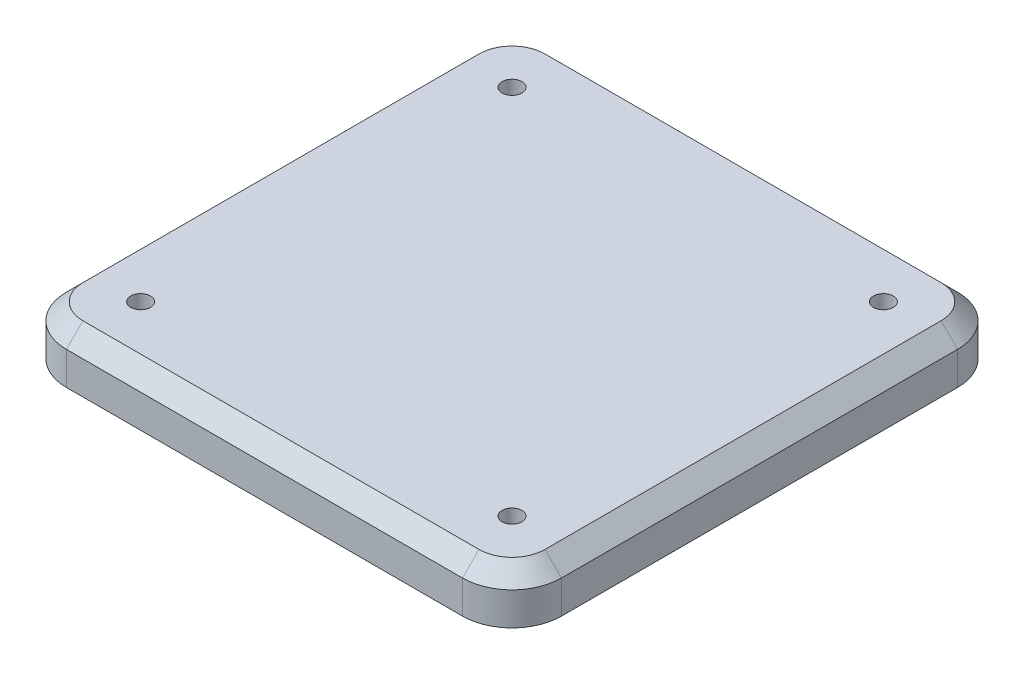
SolidWorks part; units mm, degrees
material "Plain Carbon Steel"
ref_plane "Front Plane" through (0, 0, 0) normal (0, 0, 1) x (1, 0, 0)
ref_plane "Top Plane" through (0, 0, 0) normal (0, 1, 0) x (1, 0, 0)
ref_plane "Right Plane" through (0, 0, 0) normal (1, 0, 0) x (0, 0, -1)
sketch "Base Plate Profile 300x300" plane through (0, 0, 0) normal (0, 1, 0) x (1, 0, 0)
  line L1 (-150, -150) -> (150, -150)
  line L2 (-150, -150) -> (-150, 150)
  line L3 (-150, 150) -> (150, 150)
  line L4 (150, -150) -> (150, 150)
  line L5 (-150, -150) -> (150, 150) construction
  line L6 (-150, 150) -> (150, -150) construction
  point P0 (0, 0)
  dimension "D1" = 300
  dimension "D2" = 300
extrude "Base Plate 300x300x30" add sketch "Base Plate Profile 300x300" along normal mid plane 30
fillet "Corner Fillets R30" radius 30 4 edges at (-150, 0, 150) (150, 0, 150) (-150, 0, -150) (150, 0, -150)
chamfer "Edge Chamfer 10x45" distance 10 angle 45 8 edges at (-150, 15, 0) (-141.2132, 15, 141.2132) (-141.2132, 15, -141.2132) (0, 15, 150) (0, 15, -150) (141.2132, 15, 141.2132) (141.2132, 15, -141.2132) (150, 15, 0)
sketch "Dowel Hole Layout 225 Square" plane through (0, 15, 0) normal (0, 1, 0) x (1, 0, 0)
  line L1 (-112.5, -112.5) -> (112.5, -112.5)
  line L2 (-112.5, -112.5) -> (-112.5, 112.5)
  line L3 (-112.5, 112.5) -> (112.5, 112.5)
  line L4 (112.5, -112.5) -> (112.5, 112.5)
  line L5 (-112.5, -112.5) -> (112.5, 112.5) construction
  line L6 (-112.5, 112.5) -> (112.5, -112.5) construction
  point P0 (0, 0)
  dimension "D1" = 225
  dimension "D2" = 225
hole_wizard "Dowel Holes Ø12 on 225 Square" positions "3DSketch6" profile "Sketch6" hole size "Ø12.0" standard "ANSI Metric"
sketch3d "3DSketch6"
  point P0 (112.5, 15, -112.5)
  point P3 (-112.5, 15, -112.5)
  point P6 (-112.5, 15, 112.5)
  point P9 (112.5, 15, 112.5)
sketch "Sketch6" plane through (112.5, 15, -112.5) normal (1, 0, 0) x (0, 0, 1)
  line L0 (0, 0) -> (0, 13.6052)
  line L1 (0, 13.6052) -> (6, 10)
  line L2 (6, 10) -> (6, 0)
  line L5 (6, 0) -> (0, 0)
  line L10 (0, 13.6052) -> (-6, 10) construction
  line L11 (0, -6.35) -> (0, 107.95) construction
  dimension "Hole Dia." = 12
  dimension "Hole Depth" = 10
  dimension "Drill Angle" = 118
sketch "Dowel Hole Layout 250 Square" plane through (0, -15, 0) normal (0, -1, 0) x (1, 0, 0)
  line L1 (-125, -125) -> (125, -125)
  line L2 (-125, -125) -> (-125, 125)
  line L3 (-125, 125) -> (125, 125)
  line L4 (125, -125) -> (125, 125)
  line L5 (-125, -125) -> (125, 125) construction
  line L6 (-125, 125) -> (125, -125) construction
  point P0 (0, 0)
  dimension "D1" = 250
  dimension "D2" = 250
hole_wizard "Dowel Holes Ø12 on 250 Square" positions "3DSketch7" profile "Sketch8" hole size "Ø12.0" standard "ANSI Metric"
sketch3d "3DSketch7"
  point P0 (-125, -15, 125)
  point P3 (125, -15, 125)
  point P6 (125, -15, -125)
  point P9 (-125, -15, -125)
sketch "Sketch8" plane through (-125, -15, 125) normal (1, 0, 0) x (0, 0, -1)
  line L0 (0, 0) -> (0, 13.6052)
  line L1 (0, 13.6052) -> (6, 10)
  line L2 (6, 10) -> (6, 0)
  line L5 (6, 0) -> (0, 0)
  line L10 (0, 13.6052) -> (-6, 10) construction
  line L11 (0, -6.35) -> (0, 107.95) construction
  dimension "Hole Dia." = 12
  dimension "Hole Depth" = 10
  dimension "Drill Angle" = 118
